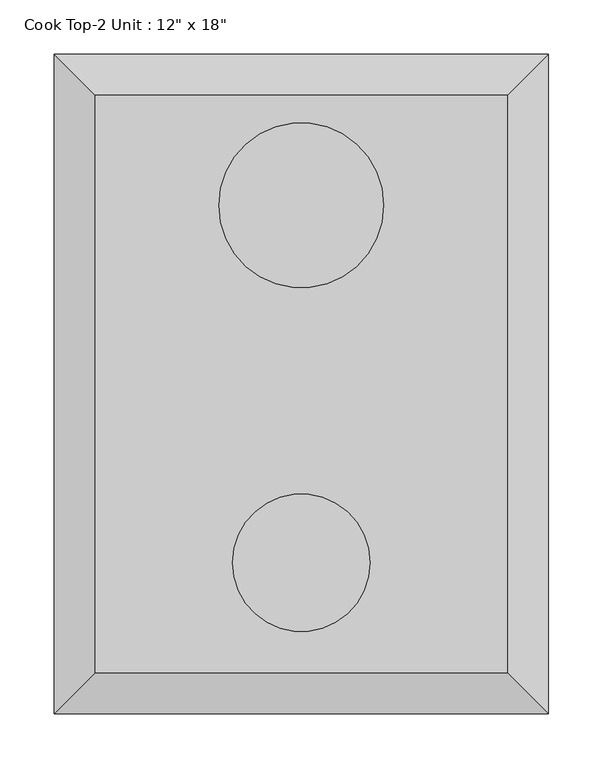
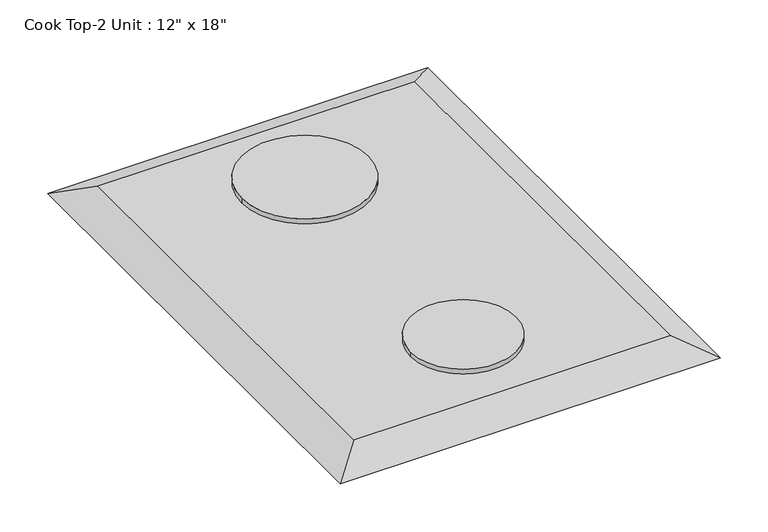
"""IFC4 building model written with IfcOpenShell, lengths in millimetres: proxy geometry."""

from ifc_helpers import new_model, si_unit, point, frame, frame_2d, origin, place, context, project, spatial, circle_curve, trimmed, segment, composite_curve, outline, extrude, faceted_brep, source, transform, mapped, element, save


def proxy_3c1fa1d0(model_context):
    return source(origin(), model_context, "Body", "SolidModel", [
        faceted_brep([(266.7, 296.9247956, 933.45), (-114.3, 296.9247956, 933.45), (-114.3, -236.4752044, 933.45), (266.7, -236.4752044, 933.45), (304.8, 335.0247956, 914.4), (304.8, -274.5752044, 914.4), (-152.4, -274.5752044, 914.4), (-152.4, 335.0247956, 914.4)], [[[0, 1, 2, 3]], [[4, 5, 6, 7]], [[4, 7, 1, 0]], [[7, 6, 2, 1]], [[6, 5, 3, 2]], [[5, 4, 0, 3]]]),
        extrude(outline(composite_curve([segment(trimmed(circle_curve(frame_2d((76.2, 195.3247956)), 76.2), [point((152.4, 195.3247956))], [point((0.0, 195.3247956))], False, "CARTESIAN"), True, "CONTINUOUS"), segment(trimmed(circle_curve(frame_2d((76.2, 195.3247956)), 76.2), [point((0.0, 195.3247956))], [point((152.4, 195.3247956))], False, "CARTESIAN"), True, "CONTINUOUS")], self_intersect=False)), frame((0.0, 0.0, 933.45), z_axis=(0.0, 0.0, 1.0), x_axis=(1.0, 0.0, 0.0)), (0.0, 0.0, 1.0), 6.35),
        extrude(outline(composite_curve([segment(trimmed(circle_curve(frame_2d((76.2, -134.8752044)), 63.5), [point((139.7, -134.8752044))], [point((12.7, -134.8752044))], False, "CARTESIAN"), True, "CONTINUOUS"), segment(trimmed(circle_curve(frame_2d((76.2, -134.8752044)), 63.5), [point((12.7, -134.8752044))], [point((139.7, -134.8752044))], False, "CARTESIAN"), True, "CONTINUOUS")], self_intersect=False)), frame((0.0, 0.0, 933.45), z_axis=(0.0, 0.0, 1.0), x_axis=(1.0, 0.0, 0.0)), (0.0, 0.0, 1.0), 6.35),
    ])


if __name__ == "__main__":
    model = new_model("IFC4")
    model_context = context("Model", 3, world=origin())
    ifc_project = project(units=[si_unit("LENGTHUNIT", "METRE", prefix="MILLI")], contexts=[model_context])
    site = spatial("IfcSite", under=ifc_project)
    building = spatial("IfcBuilding", under=site)
    placement = place(None, origin())
    proxy_shape = proxy_3c1fa1d0(model_context)
    element("IfcBuildingElementProxy", 1, Name="Cook Top-2 Unit : 12\" x 18\"", ObjectType="Cook Top-2 Unit : 12\" x 18\"", at=placement, inside=building, context=model_context, shape_type="MappedRepresentation", body=[
        mapped(proxy_shape, transform((0.0, 0.0, 0.0), x_axis=(1.0, 0.0, 0.0), y_axis=(0.0, 1.0, 0.0), z_axis=(0.0, 0.0, 1.0))),
    ])
    save(model, "model.ifc")

# Revit data of these elements
# Type "Cook Top-2 Unit : 12\" x 18\""
#   Assembly Code = "E1090400"
#   Counter Height = 3 ft
#   Depth = 2 ft
#   Width = 1.5 ft
#   Burner Material = Metal - Chrome
#   Cooktop Material = Metal - Steel, Polished
#   Default Elevation = 0
# Element 1 (IfcBuildingElementProxy, "Cook Top-2 Unit : 12\" x 18\"")
#   Materials on its faces: "Metal - Steel, Polished", "Metal - Chrome"
# Materials
#   "Metal - Chrome": class "Metal", colour RGB 247 247 247, transparency 0
#   "Metal - Steel, Polished": colour RGB 57 57 57, transparency 0
